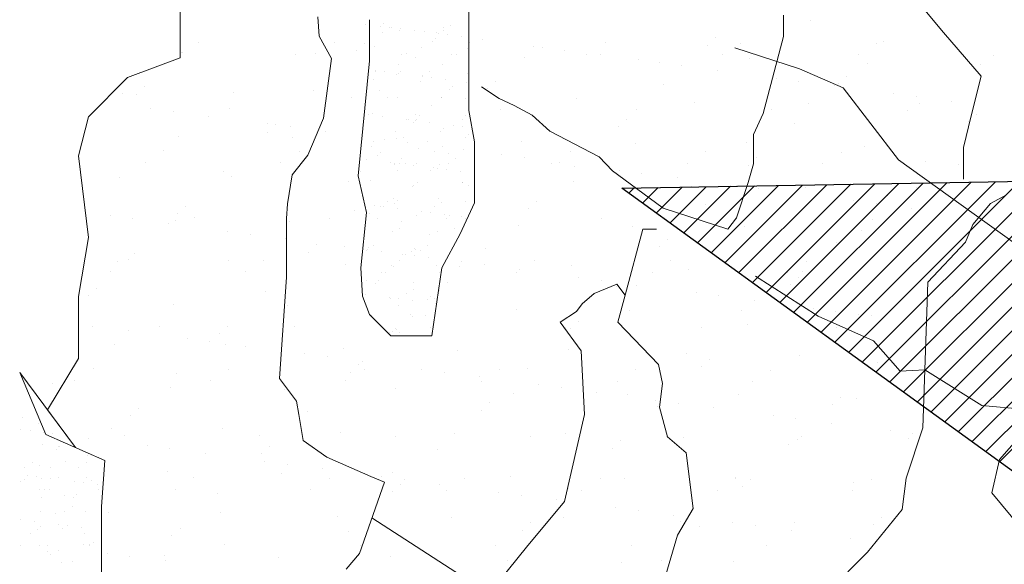
# Model space of a CAD drawing. Units: inches. Extents: x 1986 to 21484, y -1816 to 2016.
# Tile 18 of 85: x 2148.639 to 2157.681, y 1887.425 to 1892.429. Entities that reach past the tile are written whole.
import ezdxf

# ---------------------------------------------------------------- set-up
doc = ezdxf.new("R2010")
doc.units = ezdxf.units.IN
doc.layers.add('L-PLNT', color=84, linetype='Continuous', lineweight=13)
doc.layers.add('vfolha2', color=110, linetype='Continuous')

# ---------------------------------------------------------------- blocks, each defined once
blk = doc.blocks.new('arbusto_PB_verde_grande')
at = {"layer": 'vfolha2'}
h = blk.add_hatch(dxfattribs=at)
h.set_pattern_fill('ANSI31', color=256, scale=0.05, style=0)
h.set_pattern_definition([(45, (-2446.5133113, 50.986076), (-0.004419417382, 0.004419417382), [])])
h.paths.add_polyline_path([(0.02944, 0.35651), (0.00028, 0.09048), (0.02625, -0.03934), (0.047, 0.06233), (0.06189, 0.09731), (0.09372, 0.26573), (0.09955, 0.43473), (0.08789, 0.61313), (0.0645, 0.72266), (0.04988, 0.6851), (0.0236, 0.51294)])
h.paths.add_polyline_path([(0.30106, 0.43789), (0.14225, 0.24871), (0.26685, 0.30022)])
h.paths.add_polyline_path([(0.37995, 0.22817), (0.23697, 0.15193), (0.18428, 0.09364), (0.11122, 0.04358), (0.02625, -0.03934), (0.28061, 0.04667), (0.36829, 0.07798), (0.46756, 0.11239), (0.61068, 0.19376), (0.71585, 0.27823), (0.55813, 0.25948)])
h.paths.add_polyline_path([(0.56101, -0.29441), (0.72752, -0.32573), (0.59024, -0.2412), (0.42962, -0.15982), (0.02625, -0.03934), (0.14922, -0.14107), (0.18838, -0.16604), (0.41501, -0.24435)])
h.paths.add_polyline_path([(-0.27429, -0.44776), (-0.30352, -0.72628), (-0.23923, -0.64175), (-0.15457, -0.45716), (0.02625, -0.03934), (-0.16328, -0.25376)])
h.paths.add_polyline_path([(-0.51963, -0.24744), (-0.67736, -0.32573), (-0.59558, -0.35072), (-0.40574, -0.32882), (-0.21007, -0.20995), (0.02625, -0.03934), (-0.14874, -0.06595), (-0.31518, -0.09101), (-0.41452, -0.15048)])
h.paths.add_polyline_path([(-0.52546, 0.25007), (-0.70947, 0.24698), (-0.51963, 0.1093), (-0.32979, 0.02167), (-0.07567, -0.0128), (-0.04234, -0.02148), (-0.35024, 0.1312)])
for p, q in [((-0.70947, 0.24698), (-0.52546, 0.25007)), ((-0.51963, 0.1093), (-0.70947, 0.24698))]:
    blk.add_line(p, q, dxfattribs=at)
blk = doc.blocks.new('PLANT-SHRUB')
for p, q in [((2156.7576, 1892.7483), (2157.1223, 1892.3111)), ((2152.7633, 1892.5446), (2152.7633, 1892.2842)), ((2150.1112, 1892.0787), (2150.1112, 1892.4992)), ((2151.3881, 1892.279), (2151.3777, 1892.4547)), ((2151.8512, 1892.4274), (2151.8512, 1892.4274)), ((2151.8512, 1892.0499), (2151.8512, 1892.4274)), ((2155.6536, 1892.2751), (2155.6536, 1892.4702)), ((2155.9049, 1892.4263), (2155.9049, 1892.4263)), ((2151.8169, 1892.3886), (2151.8169, 1892.3886)), ((2151.9489, 1892.3658), (2151.9489, 1892.3658)), ((2151.9783, 1892.3928), (2151.9783, 1892.3928)), ((2152.0345, 1892.3568), (2152.0345, 1892.3568)), ((2152.0542, 1892.3573), (2152.0542, 1892.3573)), ((2152.1374, 1892.3464), (2152.1374, 1892.3464)), ((2152.2674, 1892.3292), (2152.2674, 1892.3292)), ((2152.5324, 1892.3559), (2152.5324, 1892.3559)), ((2152.5331, 1892.3296), (2152.5331, 1892.3296)), ((2152.598, 1892.3799), (2152.598, 1892.3799)), ((2151.5018, 1892.0724), (2151.3881, 1892.279)), ((2151.9671, 1892.3138), (2151.9671, 1892.3138)), ((2152.1241, 1892.3277), (2152.1241, 1892.3277)), ((2152.3597, 1892.3171), (2152.3597, 1892.3171)), ((2152.3597, 1892.3171), (2152.3597, 1892.3171)), ((2152.4589, 1892.2525), (2152.4589, 1892.2525)), ((2152.465, 1892.3129), (2152.465, 1892.3129)), ((2152.4845, 1892.3007), (2152.4845, 1892.3007)), ((2152.5678, 1892.2897), (2152.5678, 1892.2897)), ((2152.5678, 1892.2897), (2152.5678, 1892.2897)), ((2152.5678, 1892.2897), (2152.5678, 1892.2897)), ((2152.6977, 1892.2726), (2152.6977, 1892.2726)), ((2152.7633, 1892.2842), (2152.7633, 1891.9197)), ((2152.8927, 1892.2469), (2152.8927, 1892.2469)), ((2155.0262, 1892.2621), (2155.0262, 1892.2621)), ((2155.4666, 1891.568), (2155.6536, 1892.2751)), ((2157.1223, 1892.3111), (2157.4687, 1891.9102)), ((2150.2826, 1892.2238), (2150.2826, 1892.2238)), ((2151.5272, 1892.2215), (2151.5272, 1892.2215)), ((2151.804, 1892.213), (2151.804, 1892.213)), ((2151.8985, 1892.1851), (2151.8985, 1892.1851)), ((2152.3302, 1892.1695), (2152.3302, 1892.1695)), ((2152.4295, 1892.2255), (2152.4295, 1892.2255)), ((2152.7487, 1892.1642), (2152.7487, 1892.1642)), ((2152.7719, 1892.2192), (2152.7719, 1892.2192)), ((2153.3532, 1892.1808), (2153.3532, 1892.1808)), ((2153.4355, 1892.1755), (2153.4355, 1892.1755)), ((2153.6436, 1892.1481), (2153.6436, 1892.1481)), ((2154.0165, 1892.217), (2154.0165, 1892.217)), ((2154.9525, 1892.1946), (2154.9525, 1892.1946)), ((2155.7995, 1891.9784), (2155.2052, 1892.1705)), ((2155.2611, 1892.2147), (2155.2611, 1892.2147)), ((2156.5058, 1892.2125), (2156.5058, 1892.2125)), ((2156.5753, 1892.2299), (2156.5753, 1892.2299)), ((2149.6303, 1891.8985), (2150.1112, 1892.0787)), ((2150.114, 1892.1164), (2150.114, 1892.1164)), ((2150.1241, 1892.1256), (2150.1241, 1892.1256)), ((2150.1311, 1892.1318), (2150.1311, 1892.1318)), ((2151.1703, 1892.1123), (2151.1703, 1892.1123)), ((2151.3587, 1892.1141), (2151.3587, 1892.1141)), ((2151.4294, 1891.5247), (2151.5018, 1892.0724)), ((2151.7304, 1892.1455), (2151.7304, 1892.1455)), ((2152.1481, 1892.1111), (2152.1481, 1892.1111)), ((2152.1927, 1892.1172), (2152.1927, 1892.1172)), ((2152.1927, 1892.1172), (2152.1927, 1892.1172)), ((2152.2703, 1892.0797), (2152.2703, 1892.0797)), ((2152.6033, 1892.1119), (2152.6033, 1892.1119)), ((2152.6033, 1892.1119), (2152.6033, 1892.1119)), ((2152.646, 1892.1102), (2152.646, 1892.1102)), ((2153.2721, 1892.0783), (2153.2721, 1892.0783)), ((2153.8479, 1892.1096), (2153.8479, 1892.1096)), ((2153.9685, 1892.1053), (2153.9685, 1892.1053)), ((2154.3183, 1892.065), (2154.3183, 1892.065)), ((2155.0926, 1892.1073), (2155.0926, 1892.1073)), ((2155.3407, 1892.0699), (2155.3407, 1892.0699)), ((2156.3372, 1892.1051), (2156.3372, 1892.1051)), ((2157.5818, 1892.1028), (2157.5818, 1892.1028)), ((2151.7469, 1890.9953), (2151.8512, 1892.0499)), ((2151.8512, 1892.0499), (2151.8512, 1892.0499)), ((2152.1141, 1892.0196), (2152.1141, 1892.0196)), ((2152.523, 1892.0216), (2152.523, 1892.0216)), ((2154.5114, 1892.0338), (2154.5114, 1892.0338)), ((2154.7194, 1892.0064), (2154.7194, 1892.0064)), ((2156.2016, 1891.8037), (2155.7995, 1891.9784)), ((2156.4202, 1892.031), (2156.4202, 1892.031)), ((2157.4663, 1892.0176), (2157.4663, 1892.0176)), ((2149.2696, 1891.5381), (2149.6303, 1891.8985)), ((2151.838, 1891.9135), (2151.838, 1891.9135)), ((2151.8884, 1891.877), (2151.8884, 1891.877)), ((2151.9054, 1891.9565), (2151.9054, 1891.9565)), ((2151.9068, 1891.9628), (2151.9068, 1891.9628)), ((2151.99, 1891.9518), (2151.99, 1891.9518)), ((2152.1018, 1891.9252), (2152.1018, 1891.9252)), ((2152.12, 1891.9347), (2152.12, 1891.9347)), ((2152.1313, 1891.9522), (2152.1313, 1891.9522)), ((2152.3359, 1891.9126), (2152.3359, 1891.9126)), ((2152.3371, 1891.9061), (2152.3371, 1891.9061)), ((2152.4033, 1891.9556), (2152.4033, 1891.9556)), ((2152.4204, 1891.8952), (2152.4204, 1891.8952)), ((2152.5503, 1891.8781), (2152.5503, 1891.8781)), ((2152.7509, 1891.9394), (2152.7509, 1891.9394)), ((2152.7633, 1891.9197), (2152.7633, 1891.5942)), ((2155.0443, 1891.9637), (2155.0443, 1891.9637)), ((2155.5872, 1891.8922), (2155.5872, 1891.8922)), ((2156.2276, 1891.9113), (2156.2276, 1891.9113)), ((2157.4687, 1891.9102), (2157.3776, 1891.5458)), ((2149.7834, 1891.8131), (2149.7834, 1891.8131)), ((2152.3202, 1891.8615), (2152.3202, 1891.8615)), ((2152.6118, 1891.8119), (2152.6118, 1891.8119)), ((2152.7386, 1891.8561), (2152.7386, 1891.8561)), ((2152.8799, 1891.8118), (2153.0426, 1891.7062)), ((2152.9318, 1891.7947), (2152.9318, 1891.7947)), ((2153.0055, 1891.8622), (2153.0055, 1891.8622)), ((2154.5547, 1891.8301), (2154.5547, 1891.8301)), ((2155.7952, 1891.8648), (2155.7952, 1891.8648)), ((2156.1202, 1891.822), (2156.1202, 1891.822)), ((2156.1539, 1891.8438), (2156.1539, 1891.8438)), ((2156.7085, 1891.14), (2156.2016, 1891.8037)), ((2149.5837, 1891.7509), (2149.5837, 1891.7509)), ((2149.7097, 1891.7456), (2149.7097, 1891.7456)), ((2150.6061, 1891.7558), (2150.6061, 1891.7558)), ((2151.3326, 1891.781), (2151.3326, 1891.781)), ((2151.6855, 1891.7169), (2151.6855, 1891.7169)), ((2151.9427, 1891.7794), (2151.9427, 1891.7794)), ((2152.019, 1891.7107), (2152.019, 1891.7107)), ((2152.104, 1891.7116), (2152.104, 1891.7116)), ((2152.513, 1891.7135), (2152.513, 1891.7135)), ((2152.5169, 1891.7098), (2152.5169, 1891.7098)), ((2152.5824, 1891.7849), (2152.5824, 1891.7849)), ((2152.7317, 1891.7036), (2152.7317, 1891.7036)), ((2152.7317, 1891.7036), (2152.7317, 1891.7036)), ((2153.0426, 1891.7062), (2153.1809, 1891.6411)), ((2153.7541, 1891.7085), (2153.7541, 1891.7085)), ((2156.663, 1891.7506), (2156.663, 1891.7506)), ((2156.8711, 1891.7232), (2156.8711, 1891.7232)), ((2149.8396, 1891.6141), (2149.8396, 1891.6141)), ((2150.5665, 1891.6095), (2150.5665, 1891.6095)), ((2151.8112, 1891.6072), (2151.8112, 1891.6072)), ((2151.8112, 1891.6072), (2151.8112, 1891.6072)), ((2152.4233, 1891.6391), (2152.4233, 1891.6391)), ((2153.0558, 1891.605), (2153.0558, 1891.605)), ((2153.1809, 1891.6411), (2153.3436, 1891.5517)), ((2154.8336, 1891.6696), (2154.8336, 1891.6696)), ((2155.8797, 1891.6562), (2155.8797, 1891.6562)), ((2156.9021, 1891.6611), (2156.9021, 1891.6611)), ((2157.196, 1891.6804), (2157.196, 1891.6804)), ((2149.1795, 1891.1777), (2149.2696, 1891.5381)), ((2150.0476, 1891.5867), (2150.0476, 1891.5867)), ((2150.3725, 1891.5439), (2150.3725, 1891.5439)), ((2151.2847, 1891.1837), (2151.4294, 1891.5247)), ((2151.8426, 1891.5573), (2151.8426, 1891.5573)), ((2151.8783, 1891.569), (2151.8783, 1891.569)), ((2151.9726, 1891.5402), (2151.9726, 1891.5402)), ((2152.2742, 1891.5552), (2152.2742, 1891.5552)), ((2152.3101, 1891.5534), (2152.3101, 1891.5534)), ((2152.7286, 1891.5481), (2152.7286, 1891.5481)), ((2152.7633, 1891.5942), (2152.8154, 1891.3077)), ((2153.3436, 1891.5517), (2153.5062, 1891.4054)), ((2154.3004, 1891.6027), (2154.3004, 1891.6027)), ((2155.3771, 1891.3729), (2155.4666, 1891.568)), ((2155.5451, 1891.6004), (2155.5451, 1891.6004)), ((2156.7897, 1891.5982), (2156.7897, 1891.5982)), ((2157.3776, 1891.5458), (2157.3046, 1891.2543)), ((2157.4291, 1891.5605), (2157.4291, 1891.5605)), ((2150.9154, 1891.4724), (2150.9154, 1891.4724)), ((2150.9849, 1891.4624), (2150.9849, 1891.4624)), ((2151.1234, 1891.445), (2151.1234, 1891.445)), ((2152.1897, 1891.5116), (2152.1897, 1891.5116)), ((2152.2067, 1891.5123), (2152.2067, 1891.5123)), ((2152.2547, 1891.4847), (2152.2547, 1891.4847)), ((2152.273, 1891.5007), (2152.273, 1891.5007)), ((2152.2842, 1891.5117), (2152.2842, 1891.5117)), ((2152.4029, 1891.4836), (2152.4029, 1891.4836)), ((2152.534, 1891.4302), (2152.534, 1891.4302)), ((2152.534, 1891.4302), (2152.534, 1891.4302)), ((2152.6201, 1891.455), (2152.6201, 1891.455)), ((2152.7033, 1891.444), (2152.7033, 1891.444)), ((2152.7046, 1891.5114), (2152.7046, 1891.5114)), ((2154.1333, 1891.4439), (2154.1333, 1891.4439)), ((2154.207, 1891.5114), (2154.207, 1891.5114)), ((2155.7561, 1891.4793), (2155.7561, 1891.4793)), ((2157.3554, 1891.493), (2157.3554, 1891.493)), ((2150.0989, 1891.3555), (2150.0989, 1891.3555)), ((2150.9112, 1891.3949), (2150.9112, 1891.3949)), ((2151.1451, 1891.3422), (2151.1451, 1891.3422)), ((2151.4484, 1891.4023), (2151.4484, 1891.4023)), ((2152.0939, 1891.4035), (2152.0939, 1891.4035)), ((2152.0956, 1891.3388), (2152.0956, 1891.3388)), ((2152.1675, 1891.3471), (2152.1675, 1891.3471)), ((2152.1675, 1891.3471), (2152.1675, 1891.3471)), ((2152.5029, 1891.4055), (2152.5029, 1891.4055)), ((2152.7353, 1891.3443), (2152.7353, 1891.3443)), ((2152.7648, 1891.3713), (2152.7648, 1891.3713)), ((2153.5062, 1891.4054), (2153.9617, 1891.1697)), ((2155.3771, 1891.1047), (2155.3771, 1891.3729)), ((2151.8682, 1891.261), (2151.8682, 1891.261)), ((2151.8899, 1891.3104), (2151.8899, 1891.3104)), ((2151.9912, 1891.3308), (2151.9912, 1891.3308)), ((2151.9912, 1891.3308), (2151.9912, 1891.3308)), ((2152.1993, 1891.3034), (2152.1993, 1891.3034)), ((2152.1993, 1891.3034), (2152.1993, 1891.3034)), ((2152.3, 1891.2454), (2152.3, 1891.2454)), ((2152.3877, 1891.3095), (2152.3877, 1891.3095)), ((2152.5242, 1891.2606), (2152.5242, 1891.2606)), ((2152.5242, 1891.2606), (2152.5242, 1891.2606)), ((2152.8154, 1891.3077), (2152.8154, 1890.7479)), ((2153.247, 1891.3082), (2153.247, 1891.3082)), ((2154.2931, 1891.2949), (2154.2931, 1891.2949)), ((2155.3155, 1891.2998), (2155.3155, 1891.2998)), ((2156.395, 1891.2609), (2156.395, 1891.2609)), ((2157.3046, 1891.2543), (2157.3046, 1890.9628)), ((2149.2696, 1890.4268), (2149.1795, 1891.1777)), ((2149.9598, 1891.2229), (2149.9598, 1891.2229)), ((2151.1399, 1891.0045), (2151.2847, 1891.1837)), ((2151.2044, 1891.2207), (2151.2044, 1891.2207)), ((2151.927, 1891.1844), (2151.927, 1891.1844)), ((2151.9565, 1891.2114), (2151.9565, 1891.2114)), ((2152.145, 1891.1549), (2152.145, 1891.1549)), ((2152.4491, 1891.2184), (2152.4491, 1891.2184)), ((2152.4491, 1891.2184), (2152.4491, 1891.2184)), ((2152.5762, 1891.1985), (2152.5762, 1891.1985)), ((2152.6429, 1891.154), (2152.6429, 1891.154)), ((2152.7185, 1891.2401), (2152.7185, 1891.2401)), ((2153.0671, 1891.1892), (2153.0671, 1891.1892)), ((2153.2751, 1891.1618), (2153.2751, 1891.1618)), ((2153.6937, 1891.2162), (2153.6937, 1891.2162)), ((2153.9617, 1891.1697), (2154.0838, 1891.0397)), ((2154.9383, 1891.2139), (2154.9383, 1891.2139)), ((2155.4084, 1891.1607), (2155.4084, 1891.1607)), ((2156.183, 1891.2116), (2156.183, 1891.2116)), ((2149.7913, 1891.1156), (2149.7913, 1891.1156)), ((2151.0359, 1891.1133), (2151.0359, 1891.1133)), ((2151.8252, 1891.1457), (2151.8252, 1891.1457)), ((2152.0423, 1891.1171), (2152.0423, 1891.1171)), ((2152.0776, 1891.112), (2152.0776, 1891.112)), ((2152.0839, 1891.0955), (2152.0839, 1891.0955)), ((2152.1256, 1891.1062), (2152.1256, 1891.1062)), ((2152.1863, 1891.1116), (2152.1863, 1891.1116)), ((2152.1863, 1891.1116), (2152.1863, 1891.1116)), ((2152.2555, 1891.089), (2152.2555, 1891.089)), ((2152.2805, 1891.111), (2152.2805, 1891.111)), ((2152.2805, 1891.111), (2152.2805, 1891.111)), ((2152.4371, 1891.0711), (2152.4371, 1891.0711)), ((2152.4928, 1891.0975), (2152.4928, 1891.0975)), ((2152.5755, 1891.111), (2152.5755, 1891.111)), ((2153.5252, 1891.1088), (2153.5252, 1891.1088)), ((2153.6, 1891.119), (2153.6, 1891.119)), ((2153.7355, 1891.0794), (2153.7355, 1891.0794)), ((2154.7698, 1891.1065), (2154.7698, 1891.1065)), ((2155.3283, 1890.934), (2155.3771, 1891.1047)), ((2155.3348, 1891.0932), (2155.3348, 1891.0932)), ((2156.0144, 1891.1043), (2156.0144, 1891.1043)), ((2160.1908, 1888.6391), (2156.7085, 1891.14)), ((2156.9576, 1891.1285), (2156.9576, 1891.1285)), ((2157.2591, 1891.102), (2157.2591, 1891.102)), ((2149.5585, 1890.9808), (2149.5585, 1890.9808)), ((2150.5134, 1891.0303), (2150.5134, 1891.0303)), ((2150.5809, 1890.9857), (2150.5809, 1890.9857)), ((2151.0985, 1890.7358), (2151.1399, 1891.0045)), ((2151.8251, 1890.6567), (2151.7469, 1890.9953)), ((2151.7679, 1891.0386), (2151.7679, 1891.0386)), ((2152.1127, 1891.0441), (2152.1127, 1891.0441)), ((2152.1127, 1891.0441), (2152.1127, 1891.0441)), ((2152.4076, 1891.0441), (2152.4076, 1891.0441)), ((2152.4727, 1891.0605), (2152.4727, 1891.0605)), ((2152.5559, 1891.0495), (2152.5559, 1891.0495)), ((2152.6859, 1891.0324), (2152.6859, 1891.0324)), ((2154.0838, 1891.0397), (2154.3034, 1890.8771)), ((2154.1429, 1891.0475), (2154.1429, 1891.0475)), ((2154.3509, 1891.0201), (2154.3509, 1891.0201)), ((2154.6758, 1890.9774), (2154.6758, 1890.9774)), ((2151.6604, 1890.9468), (2151.6604, 1890.9468)), ((2151.8582, 1890.9529), (2151.8582, 1890.9529)), ((2152.2485, 1890.8983), (2152.2485, 1890.8983)), ((2152.2586, 1890.9092), (2152.2586, 1890.9092)), ((2152.29, 1890.9374), (2152.29, 1890.9374)), ((2152.7065, 1890.9335), (2152.7065, 1890.9335)), ((2152.7065, 1890.9335), (2152.7065, 1890.9335)), ((2152.7084, 1890.932), (2152.7084, 1890.932)), ((2152.7565, 1890.9083), (2152.7565, 1890.9083)), ((2153.7289, 1890.9384), (2153.7289, 1890.9384)), ((2154.8084, 1890.8995), (2154.8084, 1890.8995)), ((2155.2187, 1890.9059), (2155.2187, 1890.9059)), ((2155.2225, 1890.6089), (2155.3283, 1890.934)), ((2155.8546, 1890.8861), (2155.8546, 1890.8861)), ((2156.877, 1890.8911), (2156.877, 1890.8911)), ((2154.3034, 1890.8771), (2154.5474, 1890.6983)), ((2155.4267, 1890.8785), (2155.4267, 1890.8785)), ((2155.7517, 1890.8357), (2155.7517, 1890.8357)), ((2156.6099, 1890.8099), (2156.6099, 1890.8099)), ((2157.553, 1890.7406), (2157.702, 1890.8208)), ((2150.1657, 1890.7117), (2150.1657, 1890.7117)), ((2151.0882, 1890.6014), (2151.0985, 1890.7358)), ((2151.895, 1890.7226), (2151.895, 1890.7226)), ((2151.9485, 1890.7116), (2151.9485, 1890.7116)), ((2151.9782, 1890.7116), (2151.9782, 1890.7116)), ((2152.0159, 1890.7546), (2152.0159, 1890.7546)), ((2152.0738, 1890.7875), (2152.0738, 1890.7875)), ((2152.08, 1890.7438), (2152.08, 1890.7438)), ((2152.1094, 1890.7708), (2152.1094, 1890.7708)), ((2152.4464, 1890.7107), (2152.4464, 1890.7107)), ((2152.4827, 1890.7894), (2152.4827, 1890.7894)), ((2152.5138, 1890.7537), (2152.5138, 1890.7537)), ((2152.8154, 1890.7479), (2152.6851, 1890.4614)), ((2152.7291, 1890.758), (2152.7291, 1890.758)), ((2153.3878, 1890.7608), (2153.3878, 1890.7608)), ((2154.937, 1890.7286), (2154.937, 1890.7286)), ((2156.2945, 1890.7643), (2156.2945, 1890.7643)), ((2156.5026, 1890.7369), (2156.5026, 1890.7369)), ((2156.5362, 1890.7424), (2156.5362, 1890.7424)), ((2157.3924, 1890.5458), (2157.553, 1890.7406)), ((2149.4711, 1890.6278), (2149.4711, 1890.6278)), ((2150.092, 1890.6442), (2150.092, 1890.6442)), ((2151.7149, 1890.6796), (2151.7149, 1890.6796)), ((2151.773, 1890.149), (2151.8251, 1890.6567)), ((2151.8481, 1890.6449), (2151.8481, 1890.6449)), ((2152.1081, 1890.6945), (2152.1081, 1890.6945)), ((2152.2799, 1890.6293), (2152.2799, 1890.6293)), ((2152.3253, 1890.6659), (2152.3253, 1890.6659)), ((2152.4085, 1890.655), (2152.4085, 1890.655)), ((2152.5385, 1890.6379), (2152.5385, 1890.6379)), ((2152.59, 1890.6305), (2152.59, 1890.6305)), ((2152.6984, 1890.624), (2152.6984, 1890.624)), ((2153.3141, 1890.6933), (2153.3141, 1890.6933)), ((2154.5474, 1890.6983), (2155.1412, 1890.5032)), ((2156.8275, 1890.6941), (2156.8275, 1890.6941)), ((2149.6791, 1890.6004), (2149.6791, 1890.6004)), ((2150.004, 1890.5576), (2150.004, 1890.5576)), ((2150.0737, 1890.5854), (2150.0737, 1890.5854)), ((2150.2438, 1890.6087), (2150.2438, 1890.6087)), ((2151.0882, 1890.3018), (2151.0882, 1890.6014)), ((2151.1199, 1890.5721), (2151.1199, 1890.5721)), ((2151.4884, 1890.6064), (2151.4884, 1890.6064)), ((2151.9208, 1890.598), (2151.9208, 1890.598)), ((2152.1423, 1890.577), (2152.1423, 1890.577)), ((2152.1423, 1890.577), (2152.1423, 1890.577)), ((2152.5605, 1890.6035), (2152.5605, 1890.6035)), ((2152.733, 1890.6041), (2152.733, 1890.6041)), ((2152.733, 1890.6041), (2152.733, 1890.6041)), ((2153.2218, 1890.5381), (2153.2218, 1890.5381)), ((2153.9777, 1890.6019), (2153.9777, 1890.6019)), ((2154.268, 1890.5248), (2154.268, 1890.5248)), ((2155.1412, 1890.5032), (2155.2225, 1890.6089)), ((2155.2223, 1890.5996), (2155.2223, 1890.5996)), ((2155.2904, 1890.5297), (2155.2904, 1890.5297)), ((2156.4669, 1890.5974), (2156.4669, 1890.5974)), ((2157.3236, 1890.3853), (2157.3924, 1890.5458)), ((2150.5469, 1890.4861), (2150.5469, 1890.4861)), ((2150.7549, 1890.4587), (2150.7549, 1890.4587)), ((2152.0637, 1890.4794), (2152.0637, 1890.4794)), ((2152.1295, 1890.5089), (2152.1295, 1890.5089)), ((2152.4014, 1890.4577), (2152.4014, 1890.4577)), ((2152.4727, 1890.4814), (2152.4727, 1890.4814)), ((2152.6851, 1890.4614), (2152.5157, 1890.149)), ((2152.6274, 1890.508), (2152.6274, 1890.508)), ((2152.6851, 1890.4614), (2152.6851, 1890.4614)), ((2154.1988, 1889.8984), (2154.3599, 1890.5058)), ((2154.3599, 1890.5058), (2154.4874, 1890.5058)), ((2154.3599, 1890.5058), (2154.3599, 1890.5058)), ((2156.3698, 1890.4908), (2156.3698, 1890.4908)), ((2149.1795, 1889.8862), (2149.2696, 1890.4268)), ((2151.0799, 1890.416), (2151.0799, 1890.416)), ((2151.3672, 1890.3609), (2151.3672, 1890.3609)), ((2151.6227, 1890.3445), (2151.6227, 1890.3445)), ((2151.8868, 1890.3542), (2151.8868, 1890.3542)), ((2152.3847, 1890.3533), (2152.3847, 1890.3533)), ((2154.5156, 1890.3425), (2154.5156, 1890.3425)), ((2154.5893, 1890.41), (2154.5893, 1890.41)), ((2156.1384, 1890.3779), (2156.1384, 1890.3779)), ((2156.9795, 1890.0186), (2157.3236, 1890.3853)), ((2149.6942, 1890.2797), (2149.6942, 1890.2797)), ((2151.0882, 1890.0641), (2151.0882, 1890.3018)), ((2151.2935, 1890.2934), (2151.2935, 1890.2934)), ((2151.8194, 1890.3113), (2151.8194, 1890.3113)), ((2151.8308, 1890.3171), (2151.8308, 1890.3171)), ((2151.8308, 1890.3171), (2151.8308, 1890.3171)), ((2151.8308, 1890.3171), (2151.8308, 1890.3171)), ((2151.838, 1890.3368), (2151.838, 1890.3368)), ((2151.9607, 1890.3), (2151.9607, 1890.3)), ((2152.1557, 1890.2743), (2152.1557, 1890.2743)), ((2152.1557, 1890.2743), (2152.1557, 1890.2743)), ((2152.1779, 1890.2714), (2152.1779, 1890.2714)), ((2152.2329, 1890.3033), (2152.2329, 1890.3033)), ((2152.2611, 1890.2605), (2152.2611, 1890.2605)), ((2152.2623, 1890.3303), (2152.2623, 1890.3303)), ((2152.2698, 1890.3213), (2152.2698, 1890.3213)), ((2152.3173, 1890.3104), (2152.3173, 1890.3104)), ((2152.9163, 1890.3288), (2152.9163, 1890.3288)), ((2149.5333, 1890.2107), (2149.5333, 1890.2107)), ((2149.637, 1890.2221), (2149.637, 1890.2221)), ((2150.5557, 1890.2156), (2150.5557, 1890.2156)), ((2150.8817, 1890.2199), (2150.8817, 1890.2199)), ((2151.6352, 1890.1767), (2151.6352, 1890.1767)), ((2152.0536, 1890.1714), (2152.0536, 1890.1714)), ((2152.1263, 1890.2176), (2152.1263, 1890.2176)), ((2152.1263, 1890.2176), (2152.1263, 1890.2176)), ((2152.3911, 1890.2433), (2152.3911, 1890.2433)), ((2152.4626, 1890.1734), (2152.4626, 1890.1734)), ((2152.6813, 1890.1634), (2152.6813, 1890.1634)), ((2152.6986, 1890.2029), (2152.6986, 1890.2029)), ((2152.9066, 1890.1755), (2152.9066, 1890.1755)), ((2153.3709, 1890.2153), (2153.3709, 1890.2153)), ((2153.7037, 1890.1683), (2153.7037, 1890.1683)), ((2154.6155, 1890.2131), (2154.6155, 1890.2131)), ((2155.8602, 1890.2108), (2155.8602, 1890.2108)), ((2149.4685, 1890.1148), (2149.4685, 1890.1148)), ((2150.7131, 1890.1125), (2150.7131, 1890.1125)), ((2151.786, 1889.8886), (2151.773, 1890.149)), ((2151.9577, 1890.1102), (2151.9577, 1890.1102)), ((2151.9577, 1890.1102), (2151.9577, 1890.1102)), ((2152.0004, 1890.1085), (2152.0004, 1890.1085)), ((2152.0737, 1890.1575), (2152.0737, 1890.1575)), ((2152.5157, 1890.149), (2152.4245, 1889.524)), ((2152.4983, 1890.1076), (2152.4983, 1890.1076)), ((2153.2024, 1890.108), (2153.2024, 1890.108)), ((2153.2315, 1890.1327), (2153.2315, 1890.1327)), ((2154.447, 1890.1057), (2154.447, 1890.1057)), ((2154.7832, 1890.1294), (2154.7832, 1890.1294)), ((2155.9718, 1889.7054), (2155.3949, 1890.0722)), ((2155.6916, 1890.1034), (2155.6916, 1890.1034)), ((2155.8294, 1890.1161), (2155.8294, 1890.1161)), ((2151.0262, 1889.1313), (2151.0882, 1890.0641)), ((2151.828, 1890.0288), (2151.828, 1890.0288)), ((2151.9052, 1890.003), (2151.9052, 1890.003)), ((2151.9347, 1890.03), (2151.9347, 1890.03)), ((2152.2597, 1890.0132), (2152.2597, 1890.0132)), ((2152.5686, 1890.0102), (2152.5686, 1890.0102)), ((2153.7744, 1890.0612), (2153.7744, 1890.0612)), ((2153.9153, 1889.9136), (2154.1228, 1889.9996)), ((2153.9824, 1890.0338), (2153.9824, 1890.0338)), ((2154.1178, 1889.978), (2154.1178, 1889.978)), ((2154.1228, 1889.9996), (2154.1988, 1889.8984)), ((2154.3073, 1889.9911), (2154.3073, 1889.9911)), ((2155.7171, 1889.9917), (2155.7171, 1889.9917)), ((2155.7907, 1890.0592), (2155.7907, 1890.0592)), ((2156.968, 1889.7436), (2156.9795, 1890.0186)), ((2156.9795, 1890.0186), (2156.9795, 1890.0186)), ((2149.2728, 1889.8936), (2149.2728, 1889.8936)), ((2149.3465, 1889.9611), (2149.3465, 1889.9611)), ((2150.8957, 1889.9289), (2150.8957, 1889.9289)), ((2151.8512, 1889.7193), (2151.786, 1889.8886)), ((2151.8133, 1889.9055), (2151.8133, 1889.9055)), ((2152.1881, 1889.9101), (2152.1881, 1889.9101)), ((2152.2556, 1889.953), (2152.2556, 1889.953)), ((2152.4152, 1889.8897), (2152.4152, 1889.8897)), ((2152.4949, 1889.9427), (2152.4949, 1889.9427)), ((2153.8039, 1889.8174), (2153.9153, 1889.9136)), ((2154.1988, 1889.8984), (2154.1324, 1889.6508)), ((2154.8502, 1889.9196), (2154.8502, 1889.9196)), ((2155.0582, 1889.8922), (2155.0582, 1889.8922)), ((2149.1795, 1889.8862), (2149.1795, 1889.8862)), ((2149.1795, 1889.3156), (2149.1795, 1889.8862)), ((2150.0486, 1889.8153), (2150.0486, 1889.8153)), ((2151.0947, 1889.802), (2151.0947, 1889.802)), ((2152.0305, 1889.8769), (2152.0305, 1889.8769)), ((2152.0436, 1889.8634), (2152.0436, 1889.8634)), ((2152.1137, 1889.8659), (2152.1137, 1889.8659)), ((2152.1171, 1889.8069), (2152.1171, 1889.8069)), ((2152.1171, 1889.8069), (2152.1171, 1889.8069)), ((2152.2437, 1889.8488), (2152.2437, 1889.8488)), ((2152.3858, 1889.8627), (2152.3858, 1889.8627)), ((2152.4525, 1889.8653), (2152.4525, 1889.8653)), ((2152.4608, 1889.8202), (2152.4608, 1889.8202)), ((2153.7533, 1889.7466), (2153.8039, 1889.8174)), ((2155.3832, 1889.8494), (2155.3832, 1889.8494)), ((2152.0466, 1889.524), (2151.8512, 1889.7193)), ((2151.8713, 1889.7082), (2151.8713, 1889.7082)), ((2152.2267, 1889.7169), (2152.2267, 1889.7169)), ((2152.3691, 1889.7073), (2152.3691, 1889.7073)), ((2153.1966, 1889.768), (2153.1966, 1889.768)), ((2153.6014, 1889.6505), (2153.7533, 1889.7466)), ((2154.2428, 1889.7547), (2154.2428, 1889.7547)), ((2155.2652, 1889.7596), (2155.2652, 1889.7596)), ((2155.926, 1889.778), (2155.926, 1889.778)), ((2156.1341, 1889.7506), (2156.1341, 1889.7506)), ((2156.3446, 1889.7207), (2156.3446, 1889.7207)), ((2156.459, 1889.7078), (2156.459, 1889.7078)), ((2156.9323, 1888.68), (2156.968, 1889.7436)), ((2152.2497, 1889.7052), (2152.2497, 1889.7052)), ((2153.7961, 1889.386), (2153.6014, 1889.6505)), ((2153.7701, 1889.6594), (2153.7701, 1889.6594)), ((2154.1324, 1889.6508), (2154.5056, 1889.2597)), ((2155.3193, 1889.6272), (2155.3193, 1889.6272)), ((2156.4787, 1889.4784), (2155.9718, 1889.7054)), ((2149.3106, 1889.6141), (2149.3106, 1889.6141)), ((2149.6355, 1889.5713), (2149.6355, 1889.5713)), ((2149.921, 1889.6078), (2149.921, 1889.6078)), ((2150.4743, 1889.5428), (2150.4743, 1889.5428)), ((2150.548, 1889.6103), (2150.548, 1889.6103)), ((2151.1656, 1889.6056), (2151.1656, 1889.6056)), ((2152.0335, 1889.5553), (2152.0335, 1889.5553)), ((2152.0581, 1889.5624), (2152.0581, 1889.5624)), ((2152.0876, 1889.5894), (2152.0876, 1889.5894)), ((2152.0971, 1889.5781), (2152.0971, 1889.5781)), ((2152.0971, 1889.5781), (2152.0971, 1889.5781)), ((2152.1264, 1889.5527), (2152.1264, 1889.5527)), ((2152.4102, 1889.6033), (2152.4102, 1889.6033)), ((2152.4102, 1889.6033), (2152.4102, 1889.6033)), ((2153.6549, 1889.6011), (2153.6549, 1889.6011)), ((2153.6964, 1889.5919), (2153.6964, 1889.5919)), ((2154.8995, 1889.5988), (2154.8995, 1889.5988)), ((2156.1441, 1889.5965), (2156.1441, 1889.5965)), ((2149.5081, 1889.4406), (2149.5081, 1889.4406)), ((2150.1784, 1889.4998), (2150.1784, 1889.4998)), ((2150.3864, 1889.4725), (2150.3864, 1889.4725)), ((2150.5305, 1889.4455), (2150.5305, 1889.4455)), ((2152.0466, 1889.524), (2152.0466, 1889.524)), ((2152.4245, 1889.524), (2152.0466, 1889.524)), ((2152.4245, 1889.524), (2152.4245, 1889.524)), ((2156.7234, 1889.1989), (2156.4787, 1889.4784)), ((2150.7114, 1889.4297), (2150.7114, 1889.4297)), ((2151.2542, 1889.3582), (2151.2542, 1889.3582)), ((2151.61, 1889.4066), (2151.61, 1889.4066)), ((2152.6562, 1889.3933), (2152.6562, 1889.3933)), ((2153.6786, 1889.3982), (2153.6786, 1889.3982)), ((2153.8268, 1888.8023), (2153.7961, 1889.386)), ((2154.758, 1889.3593), (2154.758, 1889.3593)), ((2155.8042, 1889.346), (2155.8042, 1889.346)), ((2148.8944, 1888.8433), (2149.1795, 1889.3156)), ((2151.4623, 1889.3308), (2151.4623, 1889.3308)), ((2151.7494, 1889.2595), (2151.7494, 1889.2595)), ((2151.7872, 1889.288), (2151.7872, 1889.288)), ((2154.5056, 1889.2597), (2154.542, 1889.0869)), ((2154.9715, 1889.3086), (2154.9715, 1889.3086)), ((2156.5207, 1889.2764), (2156.5207, 1889.2764)), ((2148.6389, 1889.1887), (2149.1499, 1888.4979)), ((2148.6389, 1889.1887), (2148.8794, 1888.618)), ((2149.3142, 1889.2213), (2149.3142, 1889.2213)), ((2150.0765, 1889.1783), (2150.0765, 1889.1783)), ((2150.5589, 1889.219), (2150.5589, 1889.219)), ((2151.6758, 1889.192), (2151.6758, 1889.192)), ((2151.8035, 1889.2168), (2151.8035, 1889.2168)), ((2152.3301, 1889.2166), (2152.3301, 1889.2166)), ((2152.5381, 1889.1892), (2152.5381, 1889.1892)), ((2153.0481, 1889.2145), (2153.0481, 1889.2145)), ((2153.2986, 1889.2274), (2153.2986, 1889.2274)), ((2154.2928, 1889.2123), (2154.2928, 1889.2123)), ((2154.8979, 1889.2411), (2154.8979, 1889.2411)), ((2155.5374, 1889.21), (2155.5374, 1889.21)), ((2156.9502, 1889.2118), (2156.7234, 1889.1989)), ((2156.782, 1889.2077), (2156.782, 1889.2077)), ((2157.475, 1888.8845), (2156.9502, 1889.2118)), ((2148.9439, 1889.0841), (2148.9439, 1889.0841)), ((2149.1457, 1889.1139), (2149.1457, 1889.1139)), ((2150.3903, 1889.1117), (2150.3903, 1889.1117)), ((2151.0262, 1889.1313), (2151.0262, 1889.1313)), ((2151.1813, 1888.9246), (2151.0262, 1889.1313)), ((2151.635, 1889.1094), (2151.635, 1889.1094)), ((2152.863, 1889.1464), (2152.863, 1889.1464)), ((2152.8796, 1889.1072), (2152.8796, 1889.1072)), ((2153.4059, 1889.0749), (2153.4059, 1889.0749)), ((2154.1242, 1889.1049), (2154.1242, 1889.1049)), ((2154.542, 1889.0869), (2154.5147, 1888.8686)), ((2155.3689, 1889.1026), (2155.3689, 1889.1026)), ((2156.6135, 1889.1004), (2156.6135, 1889.1004)), ((2150.0234, 1889.0453), (2150.0234, 1889.0453)), ((2151.0696, 1889.0319), (2151.0696, 1889.0319)), ((2152.092, 1889.0368), (2152.092, 1889.0368)), ((2153.1714, 1888.9979), (2153.1714, 1888.9979)), ((2153.6139, 1889.0475), (2153.6139, 1889.0475)), ((2153.9388, 1889.0048), (2153.9388, 1889.0048)), ((2154.2176, 1888.9846), (2154.2176, 1888.9846)), ((2155.24, 1888.9895), (2155.24, 1888.9895)), ((2151.1813, 1888.9246), (2151.1813, 1888.9246)), ((2151.202, 1888.8006), (2151.1813, 1888.9246)), ((2152.9509, 1888.9087), (2152.9509, 1888.9087)), ((2154.4817, 1888.9333), (2154.4817, 1888.9333)), ((2154.6897, 1888.9059), (2154.6897, 1888.9059)), ((2156.173, 1888.9578), (2156.173, 1888.9578)), ((2156.3195, 1888.9506), (2156.3195, 1888.9506)), ((2148.8944, 1888.8433), (2148.8944, 1888.8433)), ((2149.1499, 1888.4979), (2148.8944, 1888.8433)), ((2149.7288, 1888.8597), (2149.7288, 1888.8597)), ((2151.278, 1888.8275), (2151.278, 1888.8275)), ((2152.8772, 1888.8412), (2152.8772, 1888.8412)), ((2153.6423, 1888.0035), (2153.8268, 1888.8023)), ((2154.5001, 1888.8766), (2154.5001, 1888.8766)), ((2154.5147, 1888.8686), (2154.5875, 1888.5957)), ((2155.0147, 1888.8631), (2155.0147, 1888.8631)), ((2156.0993, 1888.8903), (2156.0993, 1888.8903)), ((2158.0239, 1888.8339), (2157.475, 1888.8845)), ((2148.666, 1888.7769), (2148.666, 1888.7769)), ((2148.8137, 1888.7145), (2148.8137, 1888.7145)), ((2149.6551, 1888.7922), (2149.6551, 1888.7922)), ((2151.2433, 1888.563), (2151.202, 1888.8006)), ((2155.5575, 1888.7917), (2155.5575, 1888.7917)), ((2155.7656, 1888.7643), (2155.7656, 1888.7643)), ((2156.0905, 1888.7215), (2156.0905, 1888.7215)), ((2148.6418, 1888.6673), (2148.6418, 1888.6673)), ((2148.7341, 1888.6552), (2148.7341, 1888.6552)), ((2148.8589, 1888.6387), (2148.8589, 1888.6387)), ((2148.9421, 1888.6278), (2148.9421, 1888.6278)), ((2149.483, 1888.6705), (2149.483, 1888.6705)), ((2150.5054, 1888.6754), (2150.5054, 1888.6754)), ((2151.5848, 1888.6365), (2151.5848, 1888.6365)), ((2152.631, 1888.6232), (2152.631, 1888.6232)), ((2153.6534, 1888.6281), (2153.6534, 1888.6281)), ((2156.6334, 1888.65), (2156.6334, 1888.65)), ((2156.7781, 1888.2176), (2156.9323, 1888.68)), ((2156.8414, 1888.6226), (2156.8414, 1888.6226)), ((2157.6372, 1888.3894), (2157.9168, 1888.7107)), ((2148.8794, 1888.618), (2149.4204, 1888.3777)), ((2148.8794, 1888.618), (2148.8794, 1888.618)), ((2149.2671, 1888.585), (2149.2671, 1888.585)), ((2149.5982, 1888.607), (2149.5982, 1888.607)), ((2150.8428, 1888.6048), (2150.8428, 1888.6048)), ((2151.4605, 1888.408), (2151.2433, 1888.563)), ((2152.0875, 1888.6025), (2152.0875, 1888.6025)), ((2153.3321, 1888.6002), (2153.3321, 1888.6002)), ((2154.1524, 1888.558), (2154.1524, 1888.558)), ((2154.5767, 1888.598), (2154.5767, 1888.598)), ((2154.5875, 1888.5957), (2154.7604, 1888.4502)), ((2154.7329, 1888.5892), (2154.7329, 1888.5892)), ((2155.779, 1888.5759), (2155.779, 1888.5759)), ((2155.8214, 1888.5957), (2155.8214, 1888.5957)), ((2156.8014, 1888.5808), (2156.8014, 1888.5808)), ((2148.8502, 1888.5245), (2148.8502, 1888.5245)), ((2148.978, 1888.4821), (2148.978, 1888.4821)), ((2148.9947, 1888.5118), (2148.9947, 1888.5118)), ((2149.0075, 1888.5091), (2149.0075, 1888.5091)), ((2149.8099, 1888.5135), (2149.8099, 1888.5135)), ((2150.018, 1888.4862), (2150.018, 1888.4862)), ((2150.3429, 1888.4434), (2150.3429, 1888.4434)), ((2150.8566, 1888.4414), (2150.8566, 1888.4414)), ((2150.9303, 1888.5089), (2150.9303, 1888.5089)), ((2152.4794, 1888.4767), (2152.4794, 1888.4767)), ((2154.0787, 1888.4905), (2154.0787, 1888.4905)), ((2154.7604, 1888.4502), (2154.8241, 1887.9369)), ((2154.7604, 1888.4502), (2154.7604, 1888.4502)), ((2155.7015, 1888.5258), (2155.7015, 1888.5258)), ((2148.752, 1888.3571), (2148.752, 1888.3571)), ((2149.0563, 1888.3664), (2149.0563, 1888.3664)), ((2149.2498, 1888.3562), (2149.2498, 1888.3562)), ((2149.2573, 1888.4276), (2149.2573, 1888.4276)), ((2149.4204, 1888.3777), (2149.3904, 1887.9573)), ((2150.8857, 1888.3719), (2150.8857, 1888.3719)), ((2151.4605, 1888.408), (2151.4605, 1888.408)), ((2151.8639, 1888.2323), (2151.4605, 1888.408)), ((2157.5673, 1888.0821), (2157.6372, 1888.3894)), ((2148.6846, 1888.3142), (2148.6846, 1888.3142)), ((2148.8189, 1888.3363), (2148.8189, 1888.3363)), ((2148.9187, 1888.314), (2148.9187, 1888.314)), ((2149.1824, 1888.3133), (2149.1824, 1888.3133)), ((2149.9982, 1888.2752), (2149.9982, 1888.2752)), ((2151.0444, 1888.2618), (2151.0444, 1888.2618)), ((2151.0938, 1888.3445), (2151.0938, 1888.3445)), ((2151.4187, 1888.3017), (2151.4187, 1888.3017)), ((2152.0668, 1888.2667), (2152.0668, 1888.2667)), ((2148.6503, 1888.1818), (2148.6503, 1888.1818)), ((2148.6798, 1888.2088), (2148.6798, 1888.2088)), ((2148.7115, 1888.2442), (2148.7115, 1888.2442)), ((2148.7947, 1888.2333), (2148.7947, 1888.2333)), ((2148.8401, 1888.2165), (2148.8401, 1888.2165)), ((2148.9247, 1888.2162), (2148.9247, 1888.2162)), ((2148.9914, 1888.2205), (2148.9914, 1888.2205)), ((2149.1418, 1888.1876), (2149.1418, 1888.1876)), ((2149.2251, 1888.1766), (2149.2251, 1888.1766)), ((2149.2491, 1888.2184), (2149.2491, 1888.2184)), ((2149.2995, 1888.196), (2149.2995, 1888.196)), ((2150.2361, 1888.2182), (2150.2361, 1888.2182)), ((2151.4807, 1888.216), (2151.4807, 1888.216)), ((2151.7601, 1887.5256), (2151.9879, 1888.1806)), ((2151.9879, 1888.1806), (2151.8639, 1888.2323)), ((2151.9616, 1888.2303), (2151.9616, 1888.2303)), ((2152.1696, 1888.2029), (2152.1696, 1888.2029)), ((2152.7253, 1888.2137), (2152.7253, 1888.2137)), ((2153.1463, 1888.2278), (2153.1463, 1888.2278)), ((2153.97, 1888.2114), (2153.97, 1888.2114)), ((2154.1924, 1888.2145), (2154.1924, 1888.2145)), ((2155.2146, 1888.2092), (2155.2146, 1888.2092)), ((2155.2148, 1888.2194), (2155.2148, 1888.2194)), ((2155.3538, 1888.2072), (2155.3538, 1888.2072)), ((2156.2943, 1888.1805), (2156.2943, 1888.1805)), ((2156.4592, 1888.2069), (2156.4592, 1888.2069)), ((2156.7418, 1887.9274), (2156.7781, 1888.2176)), ((2156.7781, 1888.2176), (2156.7781, 1888.2176)), ((2148.8229, 1888.1131), (2148.8229, 1888.1131)), ((2148.8656, 1888.1114), (2148.8656, 1888.1114)), ((2148.9096, 1888.109), (2148.9096, 1888.109)), ((2149.355, 1888.1595), (2149.355, 1888.1595)), ((2149.3634, 1888.1105), (2149.3634, 1888.1105)), ((2150.0675, 1888.1109), (2150.0675, 1888.1109)), ((2151.3122, 1888.1086), (2151.3122, 1888.1086)), ((2152.0581, 1888.0906), (2152.0581, 1888.0906)), ((2152.1317, 1888.1581), (2152.1317, 1888.1581)), ((2152.4945, 1888.1601), (2152.4945, 1888.1601)), ((2152.5568, 1888.1063), (2152.5568, 1888.1063)), ((2153.0374, 1888.0886), (2153.0374, 1888.0886)), ((2153.6809, 1888.1259), (2153.6809, 1888.1259)), ((2153.8014, 1888.1041), (2153.8014, 1888.1041)), ((2155.0461, 1888.1018), (2155.0461, 1888.1018)), ((2155.2802, 1888.1397), (2155.2802, 1888.1397)), ((2156.2907, 1888.0996), (2156.2907, 1888.0996)), ((2157.8329, 1887.7609), (2157.5673, 1888.0821)), ((2148.836, 1888.0415), (2148.836, 1888.0415)), ((2149.0462, 1888.0583), (2149.0462, 1888.0583)), ((2149.1309, 1888.0415), (2149.1309, 1888.0415)), ((2149.1604, 1888.0685), (2149.1604, 1888.0685)), ((2150.4588, 1888.0769), (2150.4588, 1888.0769)), ((2153.2454, 1888.0613), (2153.2454, 1888.0613)), ((2153.2939, 1887.5837), (2153.6423, 1888.0035)), ((2153.5703, 1888.0185), (2153.5703, 1888.0185)), ((2148.8301, 1887.9084), (2148.8301, 1887.9084)), ((2149.0533, 1887.913), (2149.0533, 1887.913)), ((2149.1207, 1887.9559), (2149.1207, 1887.9559)), ((2149.239, 1887.9104), (2149.239, 1887.9104)), ((2149.3904, 1887.9573), (2149.3904, 1887.2965)), ((2149.4578, 1887.9004), (2149.4578, 1887.9004)), ((2150.4802, 1887.9053), (2150.4802, 1887.9053)), ((2154.1132, 1887.947), (2154.1132, 1887.947)), ((2154.3212, 1887.9196), (2154.3212, 1887.9196)), ((2154.8241, 1887.9369), (2154.6784, 1887.6913)), ((2156.4241, 1887.5374), (2156.7418, 1887.9274)), ((2148.6473, 1887.8388), (2148.6473, 1887.8388)), ((2148.7773, 1887.8216), (2148.7773, 1887.8216)), ((2148.9718, 1887.8957), (2148.9718, 1887.8957)), ((2151.5596, 1887.8664), (2151.5596, 1887.8664)), ((2151.874, 1887.8531), (2153.4137, 1886.8553)), ((2152.6058, 1887.8531), (2152.6058, 1887.8531)), ((2153.3332, 1887.8073), (2153.3332, 1887.8073)), ((2153.6282, 1887.858), (2153.6282, 1887.858)), ((2154.6462, 1887.8768), (2154.6462, 1887.8768)), ((2154.7077, 1887.8191), (2154.7077, 1887.8191)), ((2156.5553, 1887.8564), (2156.5553, 1887.8564)), ((2148.8032, 1887.7413), (2148.8032, 1887.7413)), ((2148.8327, 1887.7683), (2148.8327, 1887.7683)), ((2148.9944, 1887.7931), (2148.9944, 1887.7931)), ((2149.0362, 1887.7503), (2149.0362, 1887.7503)), ((2149.0777, 1887.7821), (2149.0777, 1887.7821)), ((2149.2076, 1887.765), (2149.2076, 1887.765)), ((2150.1111, 1887.7583), (2150.1111, 1887.7583)), ((2151.6603, 1887.7261), (2151.6603, 1887.7261)), ((2153.2595, 1887.7398), (2153.2595, 1887.7398)), ((2154.8824, 1887.7752), (2154.8824, 1887.7752)), ((2155.189, 1887.8054), (2155.189, 1887.8054)), ((2155.3971, 1887.778), (2155.3971, 1887.778)), ((2155.722, 1887.7352), (2155.722, 1887.7352)), ((2155.7539, 1887.8058), (2155.7539, 1887.8058)), ((2156.4816, 1887.7889), (2156.4816, 1887.7889)), ((2148.7365, 1887.7111), (2148.7365, 1887.7111)), ((2149.2343, 1887.7102), (2149.2343, 1887.7102)), ((2149.3133, 1887.628), (2149.3133, 1887.628)), ((2150.0374, 1887.6907), (2150.0374, 1887.6907)), ((2154.6784, 1887.6913), (2154.4964, 1887.0728)), ((2156.2649, 1887.6637), (2156.2649, 1887.6637)), ((2148.6441, 1887.5955), (2148.6441, 1887.5955)), ((2148.82, 1887.6004), (2148.82, 1887.6004)), ((2148.8936, 1887.544), (2148.8936, 1887.544)), ((2148.8986, 1887.5987), (2148.8986, 1887.5987)), ((2148.9916, 1887.5556), (2148.9916, 1887.5556)), ((2149.229, 1887.6024), (2149.229, 1887.6024)), ((2149.2754, 1887.6062), (2149.2754, 1887.6062)), ((2149.2838, 1887.601), (2149.2838, 1887.601)), ((2150.52, 1887.604), (2150.52, 1887.604)), ((2151.7647, 1887.6017), (2151.7647, 1887.6017)), ((2153.0093, 1887.5994), (2153.0093, 1887.5994)), ((2153.0377, 1887.2662), (2153.2939, 1887.5837)), ((2153.2939, 1887.5837), (2153.2939, 1887.5837)), ((2154.2539, 1887.5972), (2154.2539, 1887.5972)), ((2155.4986, 1887.5949), (2155.4986, 1887.5949)), ((2156.2426, 1887.3561), (2156.4241, 1887.5374)), ((2148.9242, 1887.5126), (2148.9242, 1887.5126)), ((2149.1247, 1887.4552), (2149.1247, 1887.4552)), ((2149.4414, 1887.5273), (2149.4414, 1887.5273)), ((2149.6495, 1887.4999), (2149.6495, 1887.4999)), ((2149.973, 1887.5051), (2149.973, 1887.5051)), ((2149.9744, 1887.4571), (2149.9744, 1887.4571)), ((2151.0192, 1887.4917), (2151.0192, 1887.4917)), ((2151.636, 1887.381), (2151.7601, 1887.5256)), ((2151.7601, 1887.5256), (2151.7601, 1887.5256)), ((2152.0416, 1887.4966), (2152.0416, 1887.4966)), ((2153.1211, 1887.4577), (2153.1211, 1887.4577)), ((2154.5346, 1887.4565), (2154.5346, 1887.4565)), ((2155.1896, 1887.4493), (2155.1896, 1887.4493)), ((2149.0261, 1887.4423), (2149.0261, 1887.4423)), ((2154.1673, 1887.4444), (2154.1673, 1887.4444))]:
    blk.add_line(p, q)

msp = doc.modelspace()

# ---------------------------------------------------------------- block references
at = {"layer": 'L-PLNT'}
msp.add_blockref('PLANT-SHRUB', (0, 0), dxfattribs=at)
at = {"layer": 'L-PLNT', "xscale": 24.60366729364114, "yscale": 24.60366729364114, "zscale": 24.60366729364114}
msp.add_blockref('arbusto_PB_verde_grande', (2171.6234, 1884.8051), dxfattribs=at)

doc.saveas('drawing.dxf')
